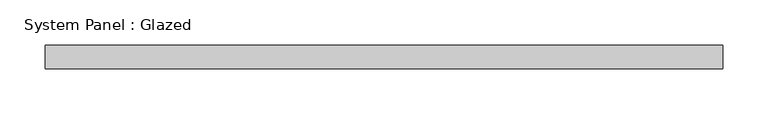
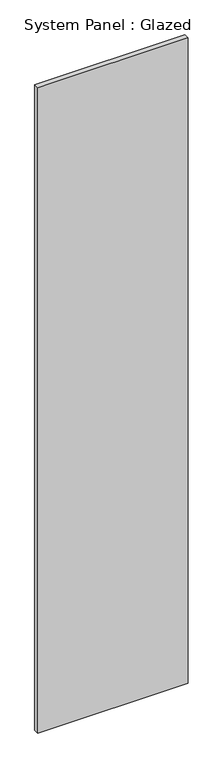
"""IFC4 building model written with IfcOpenShell, lengths in millimetres: plate geometry, System Panel : Glazed."""

from ifc_helpers import new_model, si_unit, origin, origin_with_axes, place, context, project, spatial, polyline, outline, extrude, source, transform, mapped, element, save


def system_panel_glazed_02167798(model_context):
    return source(origin(), model_context, "Body", "SweptSolid", [
        extrude(outline(polyline([(372.375, 19.05), (-372.375, 19.05), (-372.375, 44.45), (372.375, 44.45), (372.375, 19.05)])), origin_with_axes(), (0.0, 0.0, 1.0), 3379.9820397),
    ])


if __name__ == "__main__":
    model = new_model("IFC4")
    model_context = context("Model", 3, world=origin())
    ifc_project = project(units=[si_unit("LENGTHUNIT", "METRE", prefix="MILLI")], contexts=[model_context])
    site = spatial("IfcSite", under=ifc_project)
    building = spatial("IfcBuilding", under=site)
    placement = place(None, origin())
    system_panel_glazed_shape = system_panel_glazed_02167798(model_context)
    element("IfcPlate", 1, ObjectType="System Panel : Glazed", at=placement, inside=building, context=model_context, shape_type="MappedRepresentation", body=[
        mapped(system_panel_glazed_shape, transform((0.0, 0.0, 0.0), x_axis=(1.0, 0.0, 0.0), y_axis=(0.0, 1.0, 0.0), z_axis=(0.0, 0.0, 1.0))),
    ])
    save(model, "model.ifc")

# Revit data of these elements
# Type "System Panel : Glazed"
#   Construction Type Id = "GSP4R"
#   Analytic Construction = "1/8 in Pilkington single glazing"
#   Visual Light Transmittance = 0.9
#   Solar Heat Gain Coefficient = 0.86
#   Heat Transfer Coefficient (U) = 1.18115 BTU/(h·ft²·°F)
#   Define Thermal Properties by = 1
# Element 1 (IfcPlate, "System Panel : Glazed")
#   Materials on its faces: "Glass"
# Materials
#   "Glass": class "Glass", colour RGB 0 128 192, transparency 0.75, Description = "Soda Lime Glass", Cost = 0
